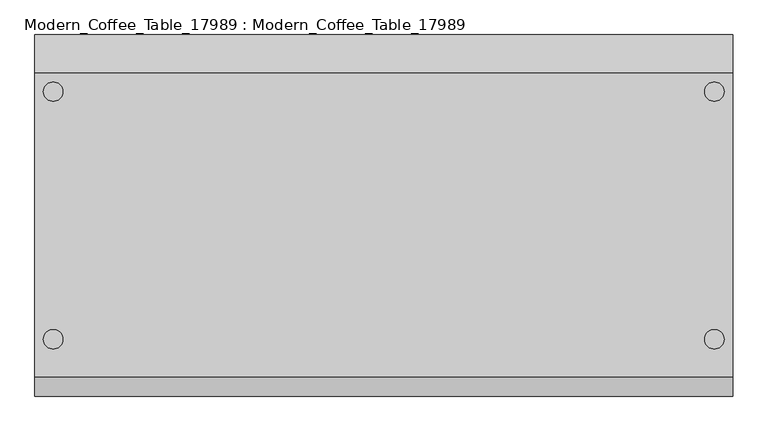
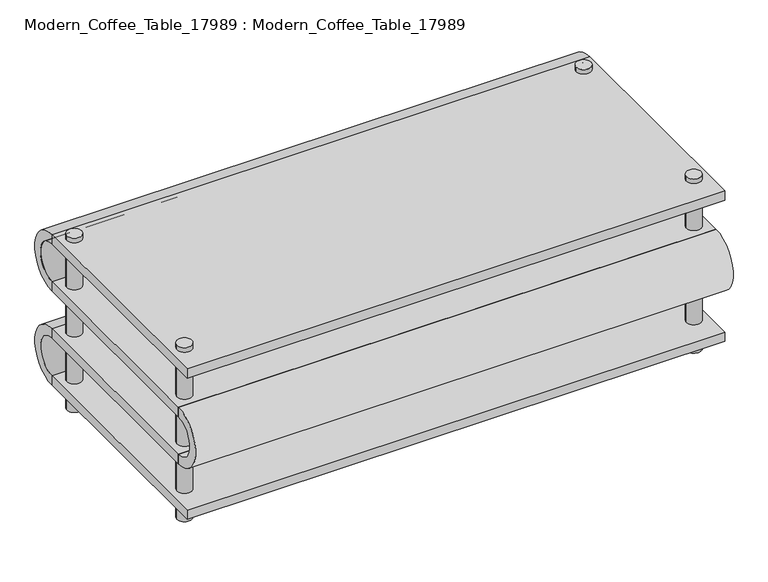
"""IFC4 building model written with IfcOpenShell, lengths in millimetres: proxy geometry, Modern_Coffee_Table_17989 : Modern_Coffee_Table_17989."""

from ifc_helpers import new_model, si_unit, point, frame, frame_2d, origin, origin_with_axes, place, context, project, spatial, polyline, circle_curve, trimmed, segment, composite_curve, outline, extrude, source, transform, mapped, element, save


def modern_coffee_table_17989_modern_coffee_table_17989_d3a860c8(model_context):
    return source(origin(), model_context, "Body", "SweptSolid", [
        extrude(outline(polyline([(457.2, -76.2), (457.2, -673.1), (-914.4, -673.1), (-914.4, -76.2), (457.2, -76.2)])), frame((0.0, 0.0, 431.8), z_axis=(0.0, 0.0, 1.0), x_axis=(1.0, 0.0, 0.0)), (0.0, 0.0, 1.0), 25.4),
        extrude(outline(polyline([(457.2, -76.2), (457.2, -673.1), (-914.4, -673.1), (-914.4, -76.2), (457.2, -76.2)])), frame((0.0, 0.0, 50.8), z_axis=(0.0, 0.0, 1.0), x_axis=(1.0, 0.0, 0.0)), (0.0, 0.0, 1.0), 25.4),
        extrude(outline(polyline([(457.2, -76.2), (457.2, -635.0), (-914.4, -635.0), (-914.4, -76.2), (457.2, -76.2)])), frame((0.0, 0.0, 304.8), z_axis=(0.0, 0.0, 1.0), x_axis=(1.0, 0.0, 0.0)), (0.0, 0.0, 1.0), 25.4),
        extrude(outline(polyline([(457.2, -76.2), (457.2, -635.0), (-914.4, -635.0), (-914.4, -76.2), (457.2, -76.2)])), frame((0.0, 0.0, 177.8), z_axis=(0.0, 0.0, 1.0), x_axis=(1.0, 0.0, 0.0)), (0.0, 0.0, 1.0), 25.4),
        extrude(outline(composite_curve([segment(trimmed(circle_curve(frame_2d((-76.2, 381.0)), 50.8), [point((-76.2, 330.2))], [point((-76.2, 431.8))], True, "CARTESIAN"), True, "CONTINUOUS"), segment(polyline([(-76.2, 431.8), (-76.2, 457.2)]), True, "CONTINUOUS"), segment(trimmed(circle_curve(frame_2d((-76.2, 381.0)), 76.2), [point((-76.2, 457.2))], [point((-76.2, 304.8))], False, "CARTESIAN"), True, "CONTINUOUS"), segment(polyline([(-76.2, 304.8), (-76.2, 330.2)]), True, "CONTINUOUS")], self_intersect=False)), frame((-914.4, 0.0, 0.0), z_axis=(1.0, 0.0, 0.0), x_axis=(0.0, 1.0, 0.0)), (0.0, 0.0, 1.0), 1371.6),
        extrude(outline(composite_curve([segment(polyline([(-635.0, 203.2), (-635.0, 177.8)]), True, "CONTINUOUS"), segment(trimmed(circle_curve(frame_2d((-635.0, 254.0)), 76.2), [point((-635.0, 177.8))], [point((-635.0, 330.2))], False, "CARTESIAN"), True, "CONTINUOUS"), segment(polyline([(-635.0, 330.2), (-635.0, 304.8)]), True, "CONTINUOUS"), segment(trimmed(circle_curve(frame_2d((-635.0, 254.0)), 50.8), [point((-635.0, 304.8))], [point((-635.0, 203.2))], True, "CARTESIAN"), True, "CONTINUOUS")], self_intersect=False)), frame((-914.4, 0.0, 0.0), z_axis=(1.0, 0.0, 0.0), x_axis=(0.0, 1.0, 0.0)), (0.0, 0.0, 1.0), 1371.6),
        extrude(outline(composite_curve([segment(trimmed(circle_curve(frame_2d((-76.2, 127.0)), 50.8), [point((-76.2, 76.2))], [point((-76.2, 177.8))], True, "CARTESIAN"), True, "CONTINUOUS"), segment(polyline([(-76.2, 177.8), (-76.2, 203.2)]), True, "CONTINUOUS"), segment(trimmed(circle_curve(frame_2d((-76.2, 127.0)), 76.2), [point((-76.2, 203.2))], [point((-76.2, 50.8))], False, "CARTESIAN"), True, "CONTINUOUS"), segment(polyline([(-76.2, 50.8), (-76.2, 76.2)]), True, "CONTINUOUS")], self_intersect=False)), frame((-914.4, 0.0, 0.0), z_axis=(1.0, 0.0, 0.0), x_axis=(0.0, 1.0, 0.0)), (0.0, 0.0, 1.0), 1371.6),
        extrude(outline(composite_curve([segment(trimmed(circle_curve(frame_2d((-878.4789755, -112.1210245)), 19.05), [point((-897.5289755, -112.1210245))], [point((-859.4289755, -112.1210245))], False, "CARTESIAN"), True, "CONTINUOUS"), segment(trimmed(circle_curve(frame_2d((-878.4789755, -112.1210245)), 19.05), [point((-859.4289755, -112.1210245))], [point((-897.5289755, -112.1210245))], False, "CARTESIAN"), True, "CONTINUOUS")], self_intersect=False)), origin_with_axes(), (0.0, 0.0, 1.0), 469.9),
        extrude(outline(composite_curve([segment(trimmed(circle_curve(frame_2d((-878.4789755, -599.0789755)), 19.05), [point((-897.5289755, -599.0789755))], [point((-859.4289755, -599.0789755))], False, "CARTESIAN"), True, "CONTINUOUS"), segment(trimmed(circle_curve(frame_2d((-878.4789755, -599.0789755)), 19.05), [point((-859.4289755, -599.0789755))], [point((-897.5289755, -599.0789755))], False, "CARTESIAN"), True, "CONTINUOUS")], self_intersect=False)), origin_with_axes(), (0.0, 0.0, 1.0), 469.9),
        extrude(outline(composite_curve([segment(trimmed(circle_curve(frame_2d((421.2789755, -599.0789755)), 19.05), [point((402.2289755, -599.0789755))], [point((440.3289755, -599.0789755))], False, "CARTESIAN"), True, "CONTINUOUS"), segment(trimmed(circle_curve(frame_2d((421.2789755, -599.0789755)), 19.05), [point((440.3289755, -599.0789755))], [point((402.2289755, -599.0789755))], False, "CARTESIAN"), True, "CONTINUOUS")], self_intersect=False)), origin_with_axes(), (0.0, 0.0, 1.0), 469.9),
        extrude(outline(composite_curve([segment(trimmed(circle_curve(frame_2d((421.2789755, -112.1210245)), 19.05), [point((402.2289755, -112.1210245))], [point((440.3289755, -112.1210245))], False, "CARTESIAN"), True, "CONTINUOUS"), segment(trimmed(circle_curve(frame_2d((421.2789755, -112.1210245)), 19.05), [point((440.3289755, -112.1210245))], [point((402.2289755, -112.1210245))], False, "CARTESIAN"), True, "CONTINUOUS")], self_intersect=False)), origin_with_axes(), (0.0, 0.0, 1.0), 469.9),
    ])


if __name__ == "__main__":
    model = new_model("IFC4")
    model_context = context("Model", 3, world=origin())
    ifc_project = project(units=[si_unit("LENGTHUNIT", "METRE", prefix="MILLI")], contexts=[model_context])
    site = spatial("IfcSite", under=ifc_project)
    building = spatial("IfcBuilding", under=site)
    placement = place(None, origin())
    modern_coffee_table_17989_modern_coffee_table_17989_shape = modern_coffee_table_17989_modern_coffee_table_17989_d3a860c8(model_context)
    element("IfcBuildingElementProxy", 1, Name="Modern_Coffee_Table_17989 : Modern_Coffee_Table_17989", ObjectType="Modern_Coffee_Table_17989 : Modern_Coffee_Table_17989", at=placement, inside=building, context=model_context, shape_type="MappedRepresentation", body=[
        mapped(modern_coffee_table_17989_modern_coffee_table_17989_shape, transform((0.0, 0.0, 0.0), x_axis=(1.0, 0.0, 0.0), y_axis=(0.0, 1.0, 0.0), z_axis=(0.0, 0.0, 1.0))),
    ])
    save(model, "model.ifc")

# Revit data of these elements
# Type "Modern_Coffee_Table_17989 : Modern_Coffee_Table_17989"
#   Default Elevation = 0
# Element 1 (IfcBuildingElementProxy, "Modern_Coffee_Table_17989 : Modern_Coffee_Table_17989")
#   Materials on its faces: "1 WOOD", "1 Glass", "1 Metal"
# Materials
#   "1 WOOD": colour RGB 32 25 15, transparency 0
#   "1 Glass": class "Glass", colour RGB 236 240 239, transparency 0.85, Cost = 0
#   "1 Metal": class "Glass", colour RGB 244 244 244, transparency 0, Cost = 0
